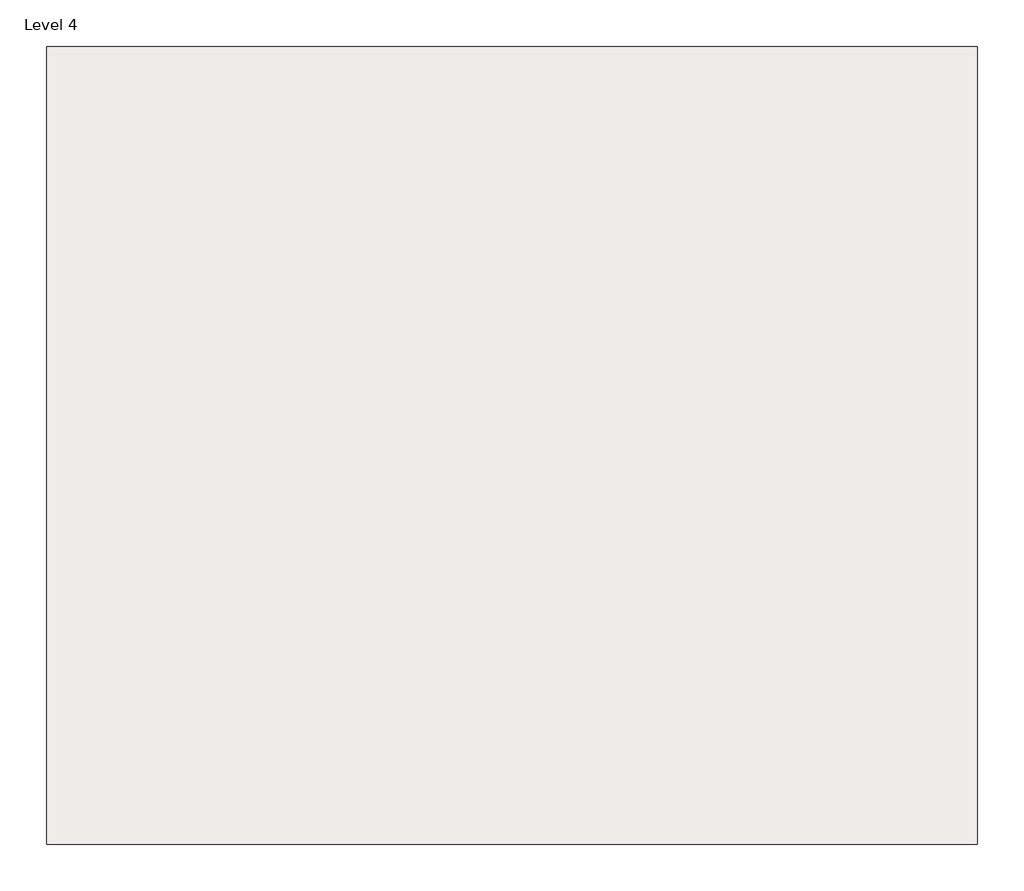
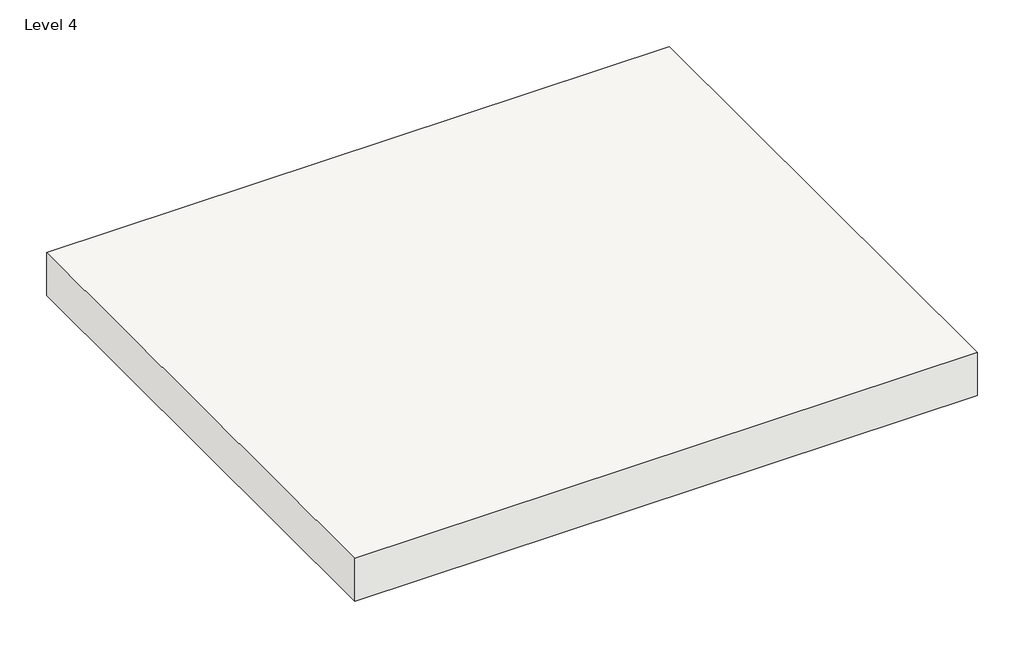
# One storey: 1 roof.
"""IFC4 building model written with IfcOpenShell, lengths in millimetres."""

from ifc_helpers import new_model, si_unit, frame, origin, place, context, project, spatial, polyline, outline, extrude, element, save

model = new_model("IFC4")

# Units and contexts
model_context = context("Model", 3, world=origin())
ifc_project = project(units=[si_unit("LENGTHUNIT", "METRE", prefix="MILLI")], contexts=[model_context])

# Site, building, storey
site = spatial("IfcSite", under=ifc_project)
building = spatial("IfcBuilding", under=site)
storey = spatial("IfcBuildingStorey", under=building, Name="Level 4", Elevation=10972.8)

# Roof
placement = place(None, origin())
element("IfcRoof", 1, ObjectType="Generic - 12\"", at=placement, inside=storey, context=model_context, shape_type="SweptSolid", body=[
    extrude(outline(polyline([(-2789.0236868, 9140.7756066), (-2789.0236868, 5546.6756066), (-6980.0236868, 5546.6756066), (-6980.0236868, 9140.7756066), (-2789.0236868, 9140.7756066)])), frame((0.0, 0.0, 10972.8), z_axis=(0.0, 0.0, 1.0), x_axis=(1.0, 0.0, 0.0)), (0.0, 0.0, 1.0), 304.8),
])

save(model, "model.ifc")

# Revit data of these elements
# Type "Generic - 12\""
#   Assembly Code = "B1020"
#   Layers, outside or top first: 1' - 0" no material (function 1)
# Element 1 (IfcRoof, "Generic - 12\"")
#   built-in parameter 1001705 = 37 (stored number, unit not read)
#   built-in parameter 1001710 = 33615
#   Phase Created = New Construction
#   Materials on its faces: "Default Roof"
# Materials
#   "Default Roof": colour RGB 88 101 114, transparency 0
